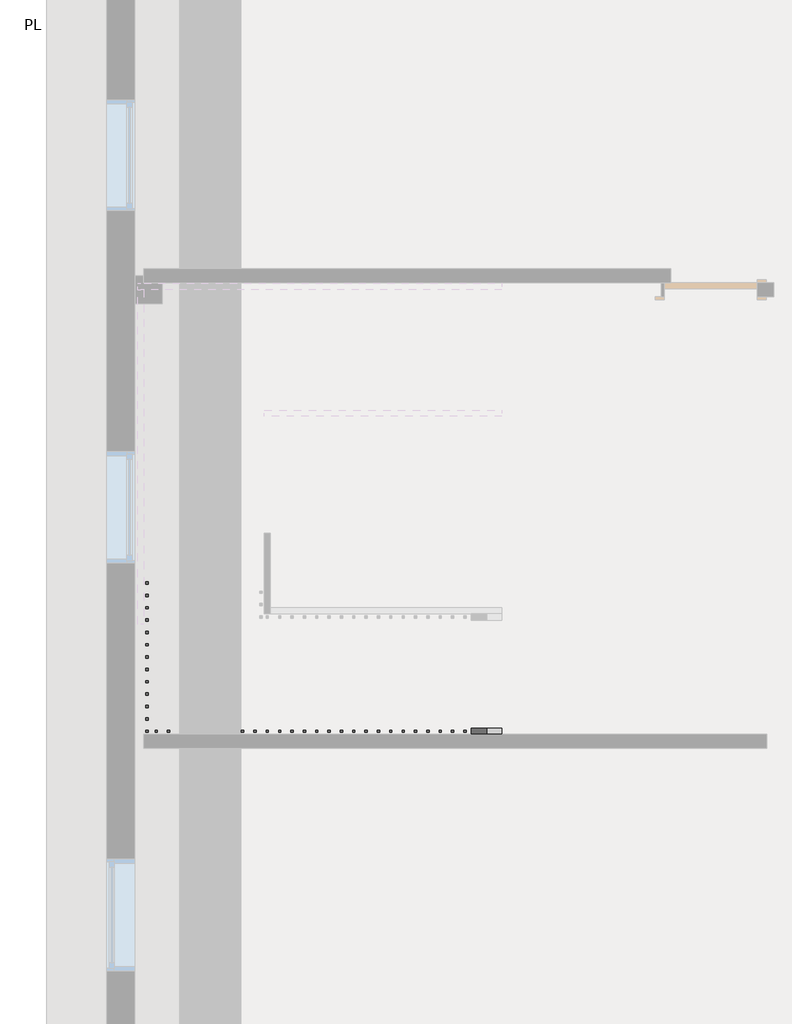
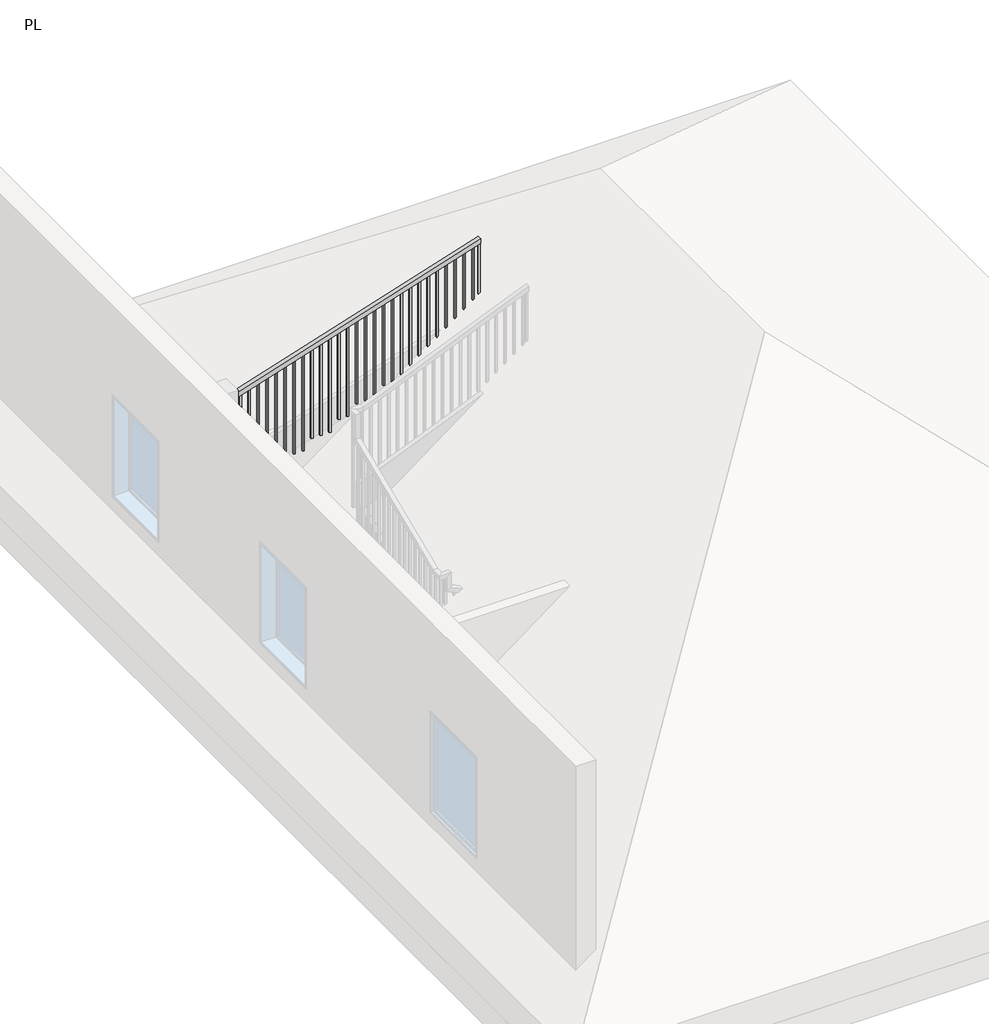
# One storey, part 2 of 3: 1 railing.
"""IFC4 building model written with IfcOpenShell, lengths in millimetres."""

from ifc_helpers import new_model, si_unit, frame, origin, place, context, project, spatial, polyline, outline, extrude, faceted_brep, element, save

model = new_model("IFC4")

# Units and contexts
model_context = context("Model", 3, world=origin())
ifc_project = project(units=[si_unit("LENGTHUNIT", "METRE", prefix="MILLI")], contexts=[model_context])

# Site, building, storey
site = spatial("IfcSite", under=ifc_project)
building = spatial("IfcBuilding", under=site)
storey = spatial("IfcBuildingStorey", under=building, Name="PL", Elevation=0.0)

# Railing
placement = place(None, origin())
element("IfcRailing", 1, ObjectType="Handrail - Rectangular", at=placement, inside=storey, context=model_context, shape_type="SolidModel", body=[
    faceted_brep([(5202.3334712, 4110.8450307, 1148.8615385), (5202.3334712, 4110.8450307, 1093.7711054), (5202.3334712, 4161.6450307, 1093.7711054), (5202.3334712, 4161.6450307, 1148.8615385), (2978.1401378, 4110.8450307, 2082.0895105), (2967.9146058, 4110.8450307, 2031.2895105), (2967.9146058, 4161.6450307, 2031.2895105), (2978.1401378, 4161.6450307, 2082.0895105), (2255.9334712, 4110.8450307, 2031.2895105), (2255.9334712, 4110.8450307, 2082.0895105), (2255.9334712, 5086.4359398, 2082.0895105), (2255.9334712, 5094.0746153, 2031.2895105), (2306.7334712, 4161.6450307, 2031.2895105), (2306.7334712, 5094.0746153, 2031.2895105), (2306.7334712, 4161.6450307, 2082.0895105), (2306.7334712, 5086.4359398, 2082.0895105), (5202.3334712, 7768.4450307, 3845.1692308), (5202.3334712, 7717.6450307, 3845.1692308), (5202.3334712, 7717.6450307, 3791.8578701), (5202.3334712, 7768.4450307, 3791.8578701), (2390.8233294, 7768.4450307, 2896.9474801), (2382.9334712, 7768.4450307, 2947.7474801), (2390.8233294, 7717.6450307, 2896.9474801), (2382.9334712, 7717.6450307, 2947.7474801), (2255.9334712, 7641.4450307, 2868.2461538), (2255.9334712, 7692.2450307, 2830.7265614), (2306.7334712, 7692.2450307, 2830.7265614), (2306.7334712, 7641.4450307, 2868.2461538), (2255.9334712, 7641.4450307, 2947.7474801), (2255.9334712, 7692.2450307, 2896.9474801), (2306.7334712, 7692.2450307, 2896.9474801), (2306.7334712, 7641.4450307, 2947.7474801), (2255.9334712, 7768.4450307, 2947.7474801), (2255.9334712, 7768.4450307, 2896.9474801), (2306.7334712, 7717.6450307, 2896.9474801), (2306.7334712, 7717.6450307, 2947.7474801)], [[[0, 1, 2, 3]], [[1, 0, 4, 5]], [[2, 1, 5, 6]], [[3, 2, 6, 7]], [[0, 3, 7, 4]], [[8, 9, 10, 11]], [[12, 8, 11, 13]], [[14, 12, 13, 15]], [[9, 14, 15, 10]], [[16, 17, 18, 19]], [[20, 21, 16, 19]], [[22, 20, 19, 18]], [[23, 22, 18, 17]], [[21, 23, 17, 16]], [[5, 4, 9, 8]], [[6, 5, 8, 12]], [[7, 6, 12, 14]], [[4, 7, 14, 9]], [[11, 10, 24, 25]], [[13, 11, 25, 26]], [[15, 13, 26, 27]], [[10, 15, 27, 24]], [[25, 24, 28, 29]], [[26, 25, 29, 30]], [[27, 26, 30, 31]], [[24, 27, 31, 28]], [[29, 28, 32, 33]], [[30, 29, 33, 34]], [[31, 30, 34, 35]], [[28, 31, 35, 32]], [[33, 32, 21, 20]], [[34, 33, 20, 22]], [[35, 34, 22, 23]], [[32, 35, 23, 21]]]),
    extrude(outline(polyline([(3764.5713979, 5116.6084712), (2813.5384615, 5116.6084712), (2813.5384615, 5135.6584712), (3770.6350584, 5135.6584712), (3764.5713979, 5116.6084712)])), frame((0.0, 7733.5200307, 0.0), z_axis=(0.0, 1.0, 0.0), x_axis=(0.0, 0.0, 1.0)), (0.0, 0.0, 1.0), 19.05),
    extrude(outline(polyline([(3732.2318754, 5015.0084712), (2813.5384615, 5015.0084712), (2813.5384615, 5034.0584712), (3738.2955359, 5034.0584712), (3732.2318754, 5015.0084712)])), frame((0.0, 7733.5200307, 0.0), z_axis=(0.0, 1.0, 0.0), x_axis=(0.0, 0.0, 1.0)), (0.0, 0.0, 1.0), 19.05),
    extrude(outline(polyline([(3699.8923528, 4913.4084712), (2813.5384615, 4913.4084712), (2813.5384615, 4932.4584712), (3705.9560133, 4932.4584712), (3699.8923528, 4913.4084712)])), frame((0.0, 7733.5200307, 0.0), z_axis=(0.0, 1.0, 0.0), x_axis=(0.0, 0.0, 1.0)), (0.0, 0.0, 1.0), 19.05),
    extrude(outline(polyline([(3667.5528303, 4811.8084712), (2696.3076923, 4811.8084712), (2696.3076923, 4830.8584712), (3673.6164908, 4830.8584712), (3667.5528303, 4811.8084712)])), frame((0.0, 7733.5200307, 0.0), z_axis=(0.0, 1.0, 0.0), x_axis=(0.0, 0.0, 1.0)), (0.0, 0.0, 1.0), 19.05),
    extrude(outline(polyline([(3635.2133077, 4710.2084712), (2696.3076923, 4710.2084712), (2696.3076923, 4729.2584712), (3641.2769682, 4729.2584712), (3635.2133077, 4710.2084712)])), frame((0.0, 7733.5200307, 0.0), z_axis=(0.0, 1.0, 0.0), x_axis=(0.0, 0.0, 1.0)), (0.0, 0.0, 1.0), 19.05),
    extrude(outline(polyline([(3602.8737852, 4608.6084712), (2579.0769231, 4608.6084712), (2579.0769231, 4627.6584712), (3608.9374457, 4627.6584712), (3602.8737852, 4608.6084712)])), frame((0.0, 7733.5200307, 0.0), z_axis=(0.0, 1.0, 0.0), x_axis=(0.0, 0.0, 1.0)), (0.0, 0.0, 1.0), 19.05),
    extrude(outline(polyline([(3570.5342626, 4507.0084712), (2579.0769231, 4507.0084712), (2579.0769231, 4526.0584712), (3576.5979231, 4526.0584712), (3570.5342626, 4507.0084712)])), frame((0.0, 7733.5200307, 0.0), z_axis=(0.0, 1.0, 0.0), x_axis=(0.0, 0.0, 1.0)), (0.0, 0.0, 1.0), 19.05),
    extrude(outline(polyline([(3538.1947401, 4405.4084712), (2579.0769231, 4405.4084712), (2579.0769231, 4424.4584712), (3544.2584006, 4424.4584712), (3538.1947401, 4405.4084712)])), frame((0.0, 7733.5200307, 0.0), z_axis=(0.0, 1.0, 0.0), x_axis=(0.0, 0.0, 1.0)), (0.0, 0.0, 1.0), 19.05),
    extrude(outline(polyline([(3505.8552176, 4303.8084712), (2461.8461538, 4303.8084712), (2461.8461538, 4322.8584712), (3511.918878, 4322.8584712), (3505.8552176, 4303.8084712)])), frame((0.0, 7733.5200307, 0.0), z_axis=(0.0, 1.0, 0.0), x_axis=(0.0, 0.0, 1.0)), (0.0, 0.0, 1.0), 19.05),
    extrude(outline(polyline([(3473.515695, 4202.2084712), (2461.8461538, 4202.2084712), (2461.8461538, 4221.2584712), (3479.5793555, 4221.2584712), (3473.515695, 4202.2084712)])), frame((0.0, 7733.5200307, 0.0), z_axis=(0.0, 1.0, 0.0), x_axis=(0.0, 0.0, 1.0)), (0.0, 0.0, 1.0), 19.05),
    extrude(outline(polyline([(3441.1761725, 4100.6084712), (2461.8461538, 4100.6084712), (2461.8461538, 4119.6584712), (3447.2398329, 4119.6584712), (3441.1761725, 4100.6084712)])), frame((0.0, 7733.5200307, 0.0), z_axis=(0.0, 1.0, 0.0), x_axis=(0.0, 0.0, 1.0)), (0.0, 0.0, 1.0), 19.05),
    extrude(outline(polyline([(3408.8366499, 3999.0084712), (2344.6153846, 3999.0084712), (2344.6153846, 4018.0584712), (3414.9003104, 4018.0584712), (3408.8366499, 3999.0084712)])), frame((0.0, 7733.5200307, 0.0), z_axis=(0.0, 1.0, 0.0), x_axis=(0.0, 0.0, 1.0)), (0.0, 0.0, 1.0), 19.05),
    extrude(outline(polyline([(3376.4971274, 3897.4084712), (2344.6153846, 3897.4084712), (2344.6153846, 3916.4584712), (3382.5607878, 3916.4584712), (3376.4971274, 3897.4084712)])), frame((0.0, 7733.5200307, 0.0), z_axis=(0.0, 1.0, 0.0), x_axis=(0.0, 0.0, 1.0)), (0.0, 0.0, 1.0), 19.05),
    extrude(outline(polyline([(3344.1576048, 3795.8084712), (2344.6153846, 3795.8084712), (2344.6153846, 3814.8584712), (3350.2212653, 3814.8584712), (3344.1576048, 3795.8084712)])), frame((0.0, 7733.5200307, 0.0), z_axis=(0.0, 1.0, 0.0), x_axis=(0.0, 0.0, 1.0)), (0.0, 0.0, 1.0), 19.05),
    extrude(outline(polyline([(3311.8180823, 3694.2084712), (2227.3846154, 3694.2084712), (2227.3846154, 3713.2584712), (3317.8817427, 3713.2584712), (3311.8180823, 3694.2084712)])), frame((0.0, 7733.5200307, 0.0), z_axis=(0.0, 1.0, 0.0), x_axis=(0.0, 0.0, 1.0)), (0.0, 0.0, 1.0), 19.05),
    extrude(outline(polyline([(3279.4785597, 3592.6084712), (2227.3846154, 3592.6084712), (2227.3846154, 3611.6584712), (3285.5422202, 3611.6584712), (3279.4785597, 3592.6084712)])), frame((0.0, 7733.5200307, 0.0), z_axis=(0.0, 1.0, 0.0), x_axis=(0.0, 0.0, 1.0)), (0.0, 0.0, 1.0), 19.05),
    extrude(outline(polyline([(3247.1390372, 3491.0084712), (2110.1538462, 3491.0084712), (2110.1538462, 3510.0584712), (3253.2026977, 3510.0584712), (3247.1390372, 3491.0084712)])), frame((0.0, 7733.5200307, 0.0), z_axis=(0.0, 1.0, 0.0), x_axis=(0.0, 0.0, 1.0)), (0.0, 0.0, 1.0), 19.05),
    extrude(outline(polyline([(3214.7995146, 3389.4084712), (2110.1538462, 3389.4084712), (2110.1538462, 3408.4584712), (3220.8631751, 3408.4584712), (3214.7995146, 3389.4084712)])), frame((0.0, 7733.5200307, 0.0), z_axis=(0.0, 1.0, 0.0), x_axis=(0.0, 0.0, 1.0)), (0.0, 0.0, 1.0), 19.05),
    extrude(outline(polyline([(3182.4599921, 3287.8084712), (2110.1538462, 3287.8084712), (2110.1538462, 3306.8584712), (3188.5236526, 3306.8584712), (3182.4599921, 3287.8084712)])), frame((0.0, 7733.5200307, 0.0), z_axis=(0.0, 1.0, 0.0), x_axis=(0.0, 0.0, 1.0)), (0.0, 0.0, 1.0), 19.05),
    extrude(outline(polyline([(3150.1204695, 3186.2084712), (1992.9230769, 3186.2084712), (1992.9230769, 3205.2584712), (3156.18413, 3205.2584712), (3150.1204695, 3186.2084712)])), frame((0.0, 7733.5200307, 0.0), z_axis=(0.0, 1.0, 0.0), x_axis=(0.0, 0.0, 1.0)), (0.0, 0.0, 1.0), 19.05),
    extrude(outline(polyline([(3117.780947, 3084.6084712), (1992.9230769, 3084.6084712), (1992.9230769, 3103.6584712), (3123.8446075, 3103.6584712), (3117.780947, 3084.6084712)])), frame((0.0, 7733.5200307, 0.0), z_axis=(0.0, 1.0, 0.0), x_axis=(0.0, 0.0, 1.0)), (0.0, 0.0, 1.0), 19.05),
    extrude(outline(polyline([(3085.4414244, 2983.0084712), (1992.9230769, 2983.0084712), (1992.9230769, 3002.0584712), (3091.5050849, 3002.0584712), (3085.4414244, 2983.0084712)])), frame((0.0, 7733.5200307, 0.0), z_axis=(0.0, 1.0, 0.0), x_axis=(0.0, 0.0, 1.0)), (0.0, 0.0, 1.0), 19.05),
    extrude(outline(polyline([(3053.1019019, 2881.4084712), (1992.9230769, 2881.4084712), (1992.9230769, 2900.4584712), (3059.1655624, 2900.4584712), (3053.1019019, 2881.4084712)])), frame((0.0, 7733.5200307, 0.0), z_axis=(0.0, 1.0, 0.0), x_axis=(0.0, 0.0, 1.0)), (0.0, 0.0, 1.0), 19.05),
    extrude(outline(polyline([(3020.7623794, 2779.8084712), (1992.9230769, 2779.8084712), (1992.9230769, 2798.8584712), (3026.8260398, 2798.8584712), (3020.7623794, 2779.8084712)])), frame((0.0, 7733.5200307, 0.0), z_axis=(0.0, 1.0, 0.0), x_axis=(0.0, 0.0, 1.0)), (0.0, 0.0, 1.0), 19.05),
    extrude(outline(polyline([(2988.4228568, 2678.2084712), (1992.9230769, 2678.2084712), (1992.9230769, 2697.2584712), (2994.4865173, 2697.2584712), (2988.4228568, 2678.2084712)])), frame((0.0, 7733.5200307, 0.0), z_axis=(0.0, 1.0, 0.0), x_axis=(0.0, 0.0, 1.0)), (0.0, 0.0, 1.0), 19.05),
    extrude(outline(polyline([(2956.0833343, 2576.6084712), (1992.9230769, 2576.6084712), (1992.9230769, 2595.6584712), (2962.1469947, 2595.6584712), (2956.0833343, 2576.6084712)])), frame((0.0, 7733.5200307, 0.0), z_axis=(0.0, 1.0, 0.0), x_axis=(0.0, 0.0, 1.0)), (0.0, 0.0, 1.0), 19.05),
    extrude(outline(polyline([(2923.7438117, 2475.0084712), (1992.9230769, 2475.0084712), (1992.9230769, 2494.0584712), (2929.8074722, 2494.0584712), (2923.7438117, 2475.0084712)])), frame((0.0, 7733.5200307, 0.0), z_axis=(0.0, 1.0, 0.0), x_axis=(0.0, 0.0, 1.0)), (0.0, 0.0, 1.0), 19.05),
    extrude(outline(polyline([(2891.4042892, 2373.4084712), (1992.9230769, 2373.4084712), (1992.9230769, 2392.4584712), (2897.4679496, 2392.4584712), (2891.4042892, 2373.4084712)])), frame((0.0, 7733.5200307, 0.0), z_axis=(0.0, 1.0, 0.0), x_axis=(0.0, 0.0, 1.0)), (0.0, 0.0, 1.0), 19.05),
    extrude(outline(polyline([(2271.8084712, 7682.7200307), (2271.8084712, 7701.7700307), (2290.8584712, 7701.7700307), (2290.8584712, 7682.7200307), (2271.8084712, 7682.7200307)])), frame((0.0, 0.0, 1875.6923077), z_axis=(0.0, 0.0, 1.0), x_axis=(1.0, 0.0, 0.0)), (0.0, 0.0, 1.0), 1021.2551724),
    extrude(outline(polyline([(7600.1700307, 2802.3957922), (7600.1700307, 1875.6923077), (7581.1200307, 1875.6923077), (7581.1200307, 2796.5342537), (7600.1700307, 2802.3957922)])), frame((2271.8084712, 0.0, 0.0), z_axis=(1.0, 0.0, 0.0), x_axis=(0.0, 1.0, 0.0)), (0.0, 0.0, 1.0), 19.05),
    extrude(outline(polyline([(7498.5700307, 2771.1342537), (7498.5700307, 1875.6923077), (7479.5200307, 1875.6923077), (7479.5200307, 2765.2727152), (7498.5700307, 2771.1342537)])), frame((2271.8084712, 0.0, 0.0), z_axis=(1.0, 0.0, 0.0), x_axis=(0.0, 1.0, 0.0)), (0.0, 0.0, 1.0), 19.05),
    extrude(outline(polyline([(7396.9700307, 2739.8727152), (7396.9700307, 1875.6923077), (7377.9200307, 1875.6923077), (7377.9200307, 2734.0111768), (7396.9700307, 2739.8727152)])), frame((2271.8084712, 0.0, 0.0), z_axis=(1.0, 0.0, 0.0), x_axis=(0.0, 1.0, 0.0)), (0.0, 0.0, 1.0), 19.05),
    extrude(outline(polyline([(7295.3700307, 2708.6111768), (7295.3700307, 1875.6923077), (7276.3200307, 1875.6923077), (7276.3200307, 2702.7496383), (7295.3700307, 2708.6111768)])), frame((2271.8084712, 0.0, 0.0), z_axis=(1.0, 0.0, 0.0), x_axis=(0.0, 1.0, 0.0)), (0.0, 0.0, 1.0), 19.05),
    extrude(outline(polyline([(7193.7700307, 2677.3496383), (7193.7700307, 1875.6923077), (7174.7200307, 1875.6923077), (7174.7200307, 2671.4880999), (7193.7700307, 2677.3496383)])), frame((2271.8084712, 0.0, 0.0), z_axis=(1.0, 0.0, 0.0), x_axis=(0.0, 1.0, 0.0)), (0.0, 0.0, 1.0), 19.05),
    extrude(outline(polyline([(7092.1700307, 2646.0880999), (7092.1700307, 1875.6923077), (7073.1200307, 1875.6923077), (7073.1200307, 2640.2265614), (7092.1700307, 2646.0880999)])), frame((2271.8084712, 0.0, 0.0), z_axis=(1.0, 0.0, 0.0), x_axis=(0.0, 1.0, 0.0)), (0.0, 0.0, 1.0), 19.05),
    extrude(outline(polyline([(6990.5700307, 2614.8265614), (6990.5700307, 1875.6923077), (6971.5200307, 1875.6923077), (6971.5200307, 2608.9650229), (6990.5700307, 2614.8265614)])), frame((2271.8084712, 0.0, 0.0), z_axis=(1.0, 0.0, 0.0), x_axis=(0.0, 1.0, 0.0)), (0.0, 0.0, 1.0), 19.05),
    extrude(outline(polyline([(6888.9700307, 2583.5650229), (6888.9700307, 1875.6923077), (6869.9200307, 1875.6923077), (6869.9200307, 2577.7034845), (6888.9700307, 2583.5650229)])), frame((2271.8084712, 0.0, 0.0), z_axis=(1.0, 0.0, 0.0), x_axis=(0.0, 1.0, 0.0)), (0.0, 0.0, 1.0), 19.05),
    extrude(outline(polyline([(6787.3700307, 2552.3034845), (6787.3700307, 1875.6923077), (6768.3200307, 1875.6923077), (6768.3200307, 2546.441946), (6787.3700307, 2552.3034845)])), frame((2271.8084712, 0.0, 0.0), z_axis=(1.0, 0.0, 0.0), x_axis=(0.0, 1.0, 0.0)), (0.0, 0.0, 1.0), 19.05),
    extrude(outline(polyline([(6685.7700307, 2521.041946), (6685.7700307, 1758.4615385), (6666.7200307, 1758.4615385), (6666.7200307, 2515.1804076), (6685.7700307, 2521.041946)])), frame((2271.8084712, 0.0, 0.0), z_axis=(1.0, 0.0, 0.0), x_axis=(0.0, 1.0, 0.0)), (0.0, 0.0, 1.0), 19.05),
    extrude(outline(polyline([(6584.1700307, 2489.7804076), (6584.1700307, 1758.4615385), (6565.1200307, 1758.4615385), (6565.1200307, 2483.9188691), (6584.1700307, 2489.7804076)])), frame((2271.8084712, 0.0, 0.0), z_axis=(1.0, 0.0, 0.0), x_axis=(0.0, 1.0, 0.0)), (0.0, 0.0, 1.0), 19.05),
    extrude(outline(polyline([(6482.5700307, 2458.5188691), (6482.5700307, 1641.2307692), (6463.5200307, 1641.2307692), (6463.5200307, 2452.6573306), (6482.5700307, 2458.5188691)])), frame((2271.8084712, 0.0, 0.0), z_axis=(1.0, 0.0, 0.0), x_axis=(0.0, 1.0, 0.0)), (0.0, 0.0, 1.0), 19.05),
    extrude(outline(polyline([(6380.9700307, 2427.2573306), (6380.9700307, 1641.2307692), (6361.9200307, 1641.2307692), (6361.9200307, 2421.3957922), (6380.9700307, 2427.2573306)])), frame((2271.8084712, 0.0, 0.0), z_axis=(1.0, 0.0, 0.0), x_axis=(0.0, 1.0, 0.0)), (0.0, 0.0, 1.0), 19.05),
    extrude(outline(polyline([(6279.3700307, 2395.9957922), (6279.3700307, 1641.2307692), (6260.3200307, 1641.2307692), (6260.3200307, 2390.1342537), (6279.3700307, 2395.9957922)])), frame((2271.8084712, 0.0, 0.0), z_axis=(1.0, 0.0, 0.0), x_axis=(0.0, 1.0, 0.0)), (0.0, 0.0, 1.0), 19.05),
    extrude(outline(polyline([(6177.7700307, 2364.7342537), (6177.7700307, 1524.0), (6158.7200307, 1524.0), (6158.7200307, 2358.8727152), (6177.7700307, 2364.7342537)])), frame((2271.8084712, 0.0, 0.0), z_axis=(1.0, 0.0, 0.0), x_axis=(0.0, 1.0, 0.0)), (0.0, 0.0, 1.0), 19.05),
    extrude(outline(polyline([(6076.1700307, 2333.4727152), (6076.1700307, 1524.0), (6057.1200307, 1524.0), (6057.1200307, 2327.6111768), (6076.1700307, 2333.4727152)])), frame((2271.8084712, 0.0, 0.0), z_axis=(1.0, 0.0, 0.0), x_axis=(0.0, 1.0, 0.0)), (0.0, 0.0, 1.0), 19.05),
    extrude(outline(polyline([(5974.5700307, 2302.2111768), (5974.5700307, 1524.0), (5955.5200307, 1524.0), (5955.5200307, 2296.3496383), (5974.5700307, 2302.2111768)])), frame((2271.8084712, 0.0, 0.0), z_axis=(1.0, 0.0, 0.0), x_axis=(0.0, 1.0, 0.0)), (0.0, 0.0, 1.0), 19.05),
    extrude(outline(polyline([(5872.9700307, 2270.9496383), (5872.9700307, 1406.7692308), (5853.9200307, 1406.7692308), (5853.9200307, 2265.0880999), (5872.9700307, 2270.9496383)])), frame((2271.8084712, 0.0, 0.0), z_axis=(1.0, 0.0, 0.0), x_axis=(0.0, 1.0, 0.0)), (0.0, 0.0, 1.0), 19.05),
    extrude(outline(polyline([(5771.3700307, 2239.6880999), (5771.3700307, 1406.7692308), (5752.3200307, 1406.7692308), (5752.3200307, 2233.8265614), (5771.3700307, 2239.6880999)])), frame((2271.8084712, 0.0, 0.0), z_axis=(1.0, 0.0, 0.0), x_axis=(0.0, 1.0, 0.0)), (0.0, 0.0, 1.0), 19.05),
    extrude(outline(polyline([(5669.7700307, 2208.4265614), (5669.7700307, 1406.7692308), (5650.7200307, 1406.7692308), (5650.7200307, 2202.5650229), (5669.7700307, 2208.4265614)])), frame((2271.8084712, 0.0, 0.0), z_axis=(1.0, 0.0, 0.0), x_axis=(0.0, 1.0, 0.0)), (0.0, 0.0, 1.0), 19.05),
    extrude(outline(polyline([(5568.1700307, 2177.1650229), (5568.1700307, 1289.5384615), (5549.1200307, 1289.5384615), (5549.1200307, 2171.3034845), (5568.1700307, 2177.1650229)])), frame((2271.8084712, 0.0, 0.0), z_axis=(1.0, 0.0, 0.0), x_axis=(0.0, 1.0, 0.0)), (0.0, 0.0, 1.0), 19.05),
    extrude(outline(polyline([(5466.5700307, 2145.9034845), (5466.5700307, 1289.5384615), (5447.5200307, 1289.5384615), (5447.5200307, 2140.041946), (5466.5700307, 2145.9034845)])), frame((2271.8084712, 0.0, 0.0), z_axis=(1.0, 0.0, 0.0), x_axis=(0.0, 1.0, 0.0)), (0.0, 0.0, 1.0), 19.05),
    extrude(outline(polyline([(5364.9700307, 2114.641946), (5364.9700307, 1172.3076923), (5345.9200307, 1172.3076923), (5345.9200307, 2108.7804076), (5364.9700307, 2114.641946)])), frame((2271.8084712, 0.0, 0.0), z_axis=(1.0, 0.0, 0.0), x_axis=(0.0, 1.0, 0.0)), (0.0, 0.0, 1.0), 19.05),
    extrude(outline(polyline([(5263.3700307, 2083.3804076), (5263.3700307, 1172.3076923), (5244.3200307, 1172.3076923), (5244.3200307, 2077.5188691), (5263.3700307, 2083.3804076)])), frame((2271.8084712, 0.0, 0.0), z_axis=(1.0, 0.0, 0.0), x_axis=(0.0, 1.0, 0.0)), (0.0, 0.0, 1.0), 19.05),
    extrude(outline(polyline([(5161.7700307, 2052.1188691), (5161.7700307, 1172.3076923), (5142.7200307, 1172.3076923), (5142.7200307, 2046.2573306), (5161.7700307, 2052.1188691)])), frame((2271.8084712, 0.0, 0.0), z_axis=(1.0, 0.0, 0.0), x_axis=(0.0, 1.0, 0.0)), (0.0, 0.0, 1.0), 19.05),
    extrude(outline(polyline([(2271.8084712, 5041.1200307), (2271.8084712, 5060.1700307), (2290.8584712, 5060.1700307), (2290.8584712, 5041.1200307), (2271.8084712, 5041.1200307)])), frame((0.0, 0.0, 1055.0769231), z_axis=(0.0, 0.0, 1.0), x_axis=(1.0, 0.0, 0.0)), (0.0, 0.0, 1.0), 976.2125874),
    extrude(outline(polyline([(2271.8084712, 4939.5200307), (2271.8084712, 4958.5700307), (2290.8584712, 4958.5700307), (2290.8584712, 4939.5200307), (2271.8084712, 4939.5200307)])), frame((0.0, 0.0, 1055.0769231), z_axis=(0.0, 0.0, 1.0), x_axis=(1.0, 0.0, 0.0)), (0.0, 0.0, 1.0), 976.2125874),
    extrude(outline(polyline([(2271.8084712, 4837.9200307), (2271.8084712, 4856.9700307), (2290.8584712, 4856.9700307), (2290.8584712, 4837.9200307), (2271.8084712, 4837.9200307)])), frame((0.0, 0.0, 1055.0769231), z_axis=(0.0, 0.0, 1.0), x_axis=(1.0, 0.0, 0.0)), (0.0, 0.0, 1.0), 976.2125874),
    extrude(outline(polyline([(2271.8084712, 4736.3200307), (2271.8084712, 4755.3700307), (2290.8584712, 4755.3700307), (2290.8584712, 4736.3200307), (2271.8084712, 4736.3200307)])), frame((0.0, 0.0, 1055.0769231), z_axis=(0.0, 0.0, 1.0), x_axis=(1.0, 0.0, 0.0)), (0.0, 0.0, 1.0), 976.2125874),
    extrude(outline(polyline([(2271.8084712, 4634.7200307), (2271.8084712, 4653.7700307), (2290.8584712, 4653.7700307), (2290.8584712, 4634.7200307), (2271.8084712, 4634.7200307)])), frame((0.0, 0.0, 1055.0769231), z_axis=(0.0, 0.0, 1.0), x_axis=(1.0, 0.0, 0.0)), (0.0, 0.0, 1.0), 976.2125874),
    extrude(outline(polyline([(2271.8084712, 4533.1200307), (2271.8084712, 4552.1700307), (2290.8584712, 4552.1700307), (2290.8584712, 4533.1200307), (2271.8084712, 4533.1200307)])), frame((0.0, 0.0, 1055.0769231), z_axis=(0.0, 0.0, 1.0), x_axis=(1.0, 0.0, 0.0)), (0.0, 0.0, 1.0), 976.2125874),
    extrude(outline(polyline([(2271.8084712, 4431.5200307), (2271.8084712, 4450.5700307), (2290.8584712, 4450.5700307), (2290.8584712, 4431.5200307), (2271.8084712, 4431.5200307)])), frame((0.0, 0.0, 1055.0769231), z_axis=(0.0, 0.0, 1.0), x_axis=(1.0, 0.0, 0.0)), (0.0, 0.0, 1.0), 976.2125874),
    extrude(outline(polyline([(2271.8084712, 4329.9200307), (2271.8084712, 4348.9700307), (2290.8584712, 4348.9700307), (2290.8584712, 4329.9200307), (2271.8084712, 4329.9200307)])), frame((0.0, 0.0, 1055.0769231), z_axis=(0.0, 0.0, 1.0), x_axis=(1.0, 0.0, 0.0)), (0.0, 0.0, 1.0), 976.2125874),
    extrude(outline(polyline([(2271.8084712, 4228.3200307), (2271.8084712, 4247.3700307), (2290.8584712, 4247.3700307), (2290.8584712, 4228.3200307), (2271.8084712, 4228.3200307)])), frame((0.0, 0.0, 1055.0769231), z_axis=(0.0, 0.0, 1.0), x_axis=(1.0, 0.0, 0.0)), (0.0, 0.0, 1.0), 976.2125874),
    extrude(outline(polyline([(2367.0584712, 4126.7200307), (2348.0084712, 4126.7200307), (2348.0084712, 4145.7700307), (2367.0584712, 4145.7700307), (2367.0584712, 4126.7200307)])), frame((0.0, 0.0, 1055.0769231), z_axis=(0.0, 0.0, 1.0), x_axis=(1.0, 0.0, 0.0)), (0.0, 0.0, 1.0), 976.2125874),
    extrude(outline(polyline([(2468.6584712, 4126.7200307), (2449.6084712, 4126.7200307), (2449.6084712, 4145.7700307), (2468.6584712, 4145.7700307), (2468.6584712, 4126.7200307)])), frame((0.0, 0.0, 1055.0769231), z_axis=(0.0, 0.0, 1.0), x_axis=(1.0, 0.0, 0.0)), (0.0, 0.0, 1.0), 976.2125874),
    extrude(outline(polyline([(2570.2584712, 4126.7200307), (2551.2084712, 4126.7200307), (2551.2084712, 4145.7700307), (2570.2584712, 4145.7700307), (2570.2584712, 4126.7200307)])), frame((0.0, 0.0, 1055.0769231), z_axis=(0.0, 0.0, 1.0), x_axis=(1.0, 0.0, 0.0)), (0.0, 0.0, 1.0), 976.2125874),
    extrude(outline(polyline([(2671.8584712, 4126.7200307), (2652.8084712, 4126.7200307), (2652.8084712, 4145.7700307), (2671.8584712, 4145.7700307), (2671.8584712, 4126.7200307)])), frame((0.0, 0.0, 1055.0769231), z_axis=(0.0, 0.0, 1.0), x_axis=(1.0, 0.0, 0.0)), (0.0, 0.0, 1.0), 976.2125874),
    extrude(outline(polyline([(2773.4584712, 4126.7200307), (2754.4084712, 4126.7200307), (2754.4084712, 4145.7700307), (2773.4584712, 4145.7700307), (2773.4584712, 4126.7200307)])), frame((0.0, 0.0, 1055.0769231), z_axis=(0.0, 0.0, 1.0), x_axis=(1.0, 0.0, 0.0)), (0.0, 0.0, 1.0), 976.2125874),
    extrude(outline(polyline([(2875.0584712, 4126.7200307), (2856.0084712, 4126.7200307), (2856.0084712, 4145.7700307), (2875.0584712, 4145.7700307), (2875.0584712, 4126.7200307)])), frame((0.0, 0.0, 1055.0769231), z_axis=(0.0, 0.0, 1.0), x_axis=(1.0, 0.0, 0.0)), (0.0, 0.0, 1.0), 976.2125874),
    extrude(outline(polyline([(2976.6584712, 4126.7200307), (2957.6084712, 4126.7200307), (2957.6084712, 4145.7700307), (2976.6584712, 4145.7700307), (2976.6584712, 4126.7200307)])), frame((0.0, 0.0, 1055.0769231), z_axis=(0.0, 0.0, 1.0), x_axis=(1.0, 0.0, 0.0)), (0.0, 0.0, 1.0), 976.2125874),
    extrude(outline(polyline([(1992.9843922, 3059.2084712), (1055.0769231, 3059.2084712), (1055.0769231, 3078.2584712), (1984.9913852, 3078.2584712), (1992.9843922, 3059.2084712)])), frame((0.0, 4126.7200307, 0.0), z_axis=(0.0, 1.0, 0.0), x_axis=(0.0, 0.0, 1.0)), (0.0, 0.0, 1.0), 19.05),
    extrude(outline(polyline([(1950.3550215, 3160.8084712), (1055.0769231, 3160.8084712), (1055.0769231, 3179.8584712), (1942.3620145, 3179.8584712), (1950.3550215, 3160.8084712)])), frame((0.0, 4126.7200307, 0.0), z_axis=(0.0, 1.0, 0.0), x_axis=(0.0, 0.0, 1.0)), (0.0, 0.0, 1.0), 19.05),
    extrude(outline(polyline([(1907.7256509, 3262.4084712), (937.8461538, 3262.4084712), (937.8461538, 3281.4584712), (1899.7326439, 3281.4584712), (1907.7256509, 3262.4084712)])), frame((0.0, 4126.7200307, 0.0), z_axis=(0.0, 1.0, 0.0), x_axis=(0.0, 0.0, 1.0)), (0.0, 0.0, 1.0), 19.05),
    extrude(outline(polyline([(1865.0962803, 3364.0084712), (937.8461538, 3364.0084712), (937.8461538, 3383.0584712), (1857.1032733, 3383.0584712), (1865.0962803, 3364.0084712)])), frame((0.0, 4126.7200307, 0.0), z_axis=(0.0, 1.0, 0.0), x_axis=(0.0, 0.0, 1.0)), (0.0, 0.0, 1.0), 19.05),
    extrude(outline(polyline([(1822.4669096, 3465.6084712), (937.8461538, 3465.6084712), (937.8461538, 3484.6584712), (1814.4739026, 3484.6584712), (1822.4669096, 3465.6084712)])), frame((0.0, 4126.7200307, 0.0), z_axis=(0.0, 1.0, 0.0), x_axis=(0.0, 0.0, 1.0)), (0.0, 0.0, 1.0), 19.05),
    extrude(outline(polyline([(1779.837539, 3567.2084712), (820.6153846, 3567.2084712), (820.6153846, 3586.2584712), (1771.844532, 3586.2584712), (1779.837539, 3567.2084712)])), frame((0.0, 4126.7200307, 0.0), z_axis=(0.0, 1.0, 0.0), x_axis=(0.0, 0.0, 1.0)), (0.0, 0.0, 1.0), 19.05),
    extrude(outline(polyline([(1737.2081684, 3668.8084712), (820.6153846, 3668.8084712), (820.6153846, 3687.8584712), (1729.2151614, 3687.8584712), (1737.2081684, 3668.8084712)])), frame((0.0, 4126.7200307, 0.0), z_axis=(0.0, 1.0, 0.0), x_axis=(0.0, 0.0, 1.0)), (0.0, 0.0, 1.0), 19.05),
    extrude(outline(polyline([(1694.5787978, 3770.4084712), (820.6153846, 3770.4084712), (820.6153846, 3789.4584712), (1686.5857908, 3789.4584712), (1694.5787978, 3770.4084712)])), frame((0.0, 4126.7200307, 0.0), z_axis=(0.0, 1.0, 0.0), x_axis=(0.0, 0.0, 1.0)), (0.0, 0.0, 1.0), 19.05),
    extrude(outline(polyline([(1651.9494271, 3872.0084712), (703.3846154, 3872.0084712), (703.3846154, 3891.0584712), (1643.9564201, 3891.0584712), (1651.9494271, 3872.0084712)])), frame((0.0, 4126.7200307, 0.0), z_axis=(0.0, 1.0, 0.0), x_axis=(0.0, 0.0, 1.0)), (0.0, 0.0, 1.0), 19.05),
    extrude(outline(polyline([(1609.3200565, 3973.6084712), (703.3846154, 3973.6084712), (703.3846154, 3992.6584712), (1601.3270495, 3992.6584712), (1609.3200565, 3973.6084712)])), frame((0.0, 4126.7200307, 0.0), z_axis=(0.0, 1.0, 0.0), x_axis=(0.0, 0.0, 1.0)), (0.0, 0.0, 1.0), 19.05),
    extrude(outline(polyline([(1566.6906859, 4075.2084712), (703.3846154, 4075.2084712), (703.3846154, 4094.2584712), (1558.6976789, 4094.2584712), (1566.6906859, 4075.2084712)])), frame((0.0, 4126.7200307, 0.0), z_axis=(0.0, 1.0, 0.0), x_axis=(0.0, 0.0, 1.0)), (0.0, 0.0, 1.0), 19.05),
    extrude(outline(polyline([(1524.0613152, 4176.8084712), (586.1538462, 4176.8084712), (586.1538462, 4195.8584712), (1516.0683082, 4195.8584712), (1524.0613152, 4176.8084712)])), frame((0.0, 4126.7200307, 0.0), z_axis=(0.0, 1.0, 0.0), x_axis=(0.0, 0.0, 1.0)), (0.0, 0.0, 1.0), 19.05),
    extrude(outline(polyline([(1481.4319446, 4278.4084712), (586.1538462, 4278.4084712), (586.1538462, 4297.4584712), (1473.4389376, 4297.4584712), (1481.4319446, 4278.4084712)])), frame((0.0, 4126.7200307, 0.0), z_axis=(0.0, 1.0, 0.0), x_axis=(0.0, 0.0, 1.0)), (0.0, 0.0, 1.0), 19.05),
    extrude(outline(polyline([(1438.802574, 4380.0084712), (468.9230769, 4380.0084712), (468.9230769, 4399.0584712), (1430.809567, 4399.0584712), (1438.802574, 4380.0084712)])), frame((0.0, 4126.7200307, 0.0), z_axis=(0.0, 1.0, 0.0), x_axis=(0.0, 0.0, 1.0)), (0.0, 0.0, 1.0), 19.05),
    extrude(outline(polyline([(1396.1732033, 4481.6084712), (468.9230769, 4481.6084712), (468.9230769, 4500.6584712), (1388.1801964, 4500.6584712), (1396.1732033, 4481.6084712)])), frame((0.0, 4126.7200307, 0.0), z_axis=(0.0, 1.0, 0.0), x_axis=(0.0, 0.0, 1.0)), (0.0, 0.0, 1.0), 19.05),
    extrude(outline(polyline([(1353.5438327, 4583.2084712), (468.9230769, 4583.2084712), (468.9230769, 4602.2584712), (1345.5508257, 4602.2584712), (1353.5438327, 4583.2084712)])), frame((0.0, 4126.7200307, 0.0), z_axis=(0.0, 1.0, 0.0), x_axis=(0.0, 0.0, 1.0)), (0.0, 0.0, 1.0), 19.05),
    extrude(outline(polyline([(1310.9144621, 4684.8084712), (351.6923077, 4684.8084712), (351.6923077, 4703.8584712), (1302.9214551, 4703.8584712), (1310.9144621, 4684.8084712)])), frame((0.0, 4126.7200307, 0.0), z_axis=(0.0, 1.0, 0.0), x_axis=(0.0, 0.0, 1.0)), (0.0, 0.0, 1.0), 19.05),
    extrude(outline(polyline([(1268.2850915, 4786.4084712), (351.6923077, 4786.4084712), (351.6923077, 4805.4584712), (1260.2920845, 4805.4584712), (1268.2850915, 4786.4084712)])), frame((0.0, 4126.7200307, 0.0), z_axis=(0.0, 1.0, 0.0), x_axis=(0.0, 0.0, 1.0)), (0.0, 0.0, 1.0), 19.05),
    extrude(outline(polyline([(1225.6557208, 4888.0084712), (351.6923077, 4888.0084712), (351.6923077, 4907.0584712), (1217.6627138, 4907.0584712), (1225.6557208, 4888.0084712)])), frame((0.0, 4126.7200307, 0.0), z_axis=(0.0, 1.0, 0.0), x_axis=(0.0, 0.0, 1.0)), (0.0, 0.0, 1.0), 19.05),
    extrude(outline(polyline([(1183.0263502, 4989.6084712), (234.4615385, 4989.6084712), (234.4615385, 5008.6584712), (1175.0333432, 5008.6584712), (1183.0263502, 4989.6084712)])), frame((0.0, 4126.7200307, 0.0), z_axis=(0.0, 1.0, 0.0), x_axis=(0.0, 0.0, 1.0)), (0.0, 0.0, 1.0), 19.05),
    extrude(outline(polyline([(1140.3969796, 5091.2084712), (234.4615385, 5091.2084712), (234.4615385, 5110.2584712), (1132.4039726, 5110.2584712), (1140.3969796, 5091.2084712)])), frame((0.0, 4126.7200307, 0.0), z_axis=(0.0, 1.0, 0.0), x_axis=(0.0, 0.0, 1.0)), (0.0, 0.0, 1.0), 19.05),
    extrude(outline(polyline([(2271.8084712, 7733.5200307), (2271.8084712, 7752.5700307), (2290.8584712, 7752.5700307), (2290.8584712, 7733.5200307), (2271.8084712, 7733.5200307)])), frame((0.0, 0.0, 1875.6923077), z_axis=(0.0, 0.0, 1.0), x_axis=(1.0, 0.0, 0.0)), (0.0, 0.0, 1.0), 1021.2551724),
    extrude(outline(polyline([(2290.8584712, 4126.7200307), (2271.8084712, 4126.7200307), (2271.8084712, 4145.7700307), (2290.8584712, 4145.7700307), (2290.8584712, 4126.7200307)])), frame((0.0, 0.0, 1055.0769231), z_axis=(0.0, 0.0, 1.0), x_axis=(1.0, 0.0, 0.0)), (0.0, 0.0, 1.0), 976.2125874),
    extrude(outline(polyline([(3785.7942096, 5183.2834712), (2930.7692308, 5183.2834712), (2930.7692308, 5202.3334712), (3791.8578701, 5202.3334712), (3785.7942096, 5183.2834712)])), frame((0.0, 7733.5200307, 0.0), z_axis=(0.0, 1.0, 0.0), x_axis=(0.0, 0.0, 1.0)), (0.0, 0.0, 1.0), 19.05),
    extrude(outline(polyline([(1101.7641124, 5183.2834712), (117.2307692, 5183.2834712), (117.2307692, 5202.3334712), (1093.7711054, 5202.3334712), (1101.7641124, 5183.2834712)])), frame((0.0, 4126.7200307, 0.0), z_axis=(0.0, 1.0, 0.0), x_axis=(0.0, 0.0, 1.0)), (0.0, 0.0, 1.0), 19.05),
])

save(model, "model.ifc")

# Revit data of these elements
# Type "Handrail - Rectangular"
#   Assembly Code = "C2010400"
#   built-in parameter 1008612 = 0.0416667 (stored number, unit not read)
#   built-in parameter 1008611 = 0.0416667 (stored number, unit not read)
#   built-in parameter 1008609 = 0.333333 (stored number, unit not read)
#   built-in parameter 1008604 = 0.166667 (stored number, unit not read)
#   built-in parameter 1008603 = 0.166667 (stored number, unit not read)
#   Railing Height = 3' - 0"
#   built-in parameter 1008630 = 2
#   built-in parameter 1008610 = 2
#   built-in parameter 1008618 = Baluster - Square : 3/4"
# Element 1 (IfcRailing, "Handrail - Rectangular")
#   Phase Created = New Construction
